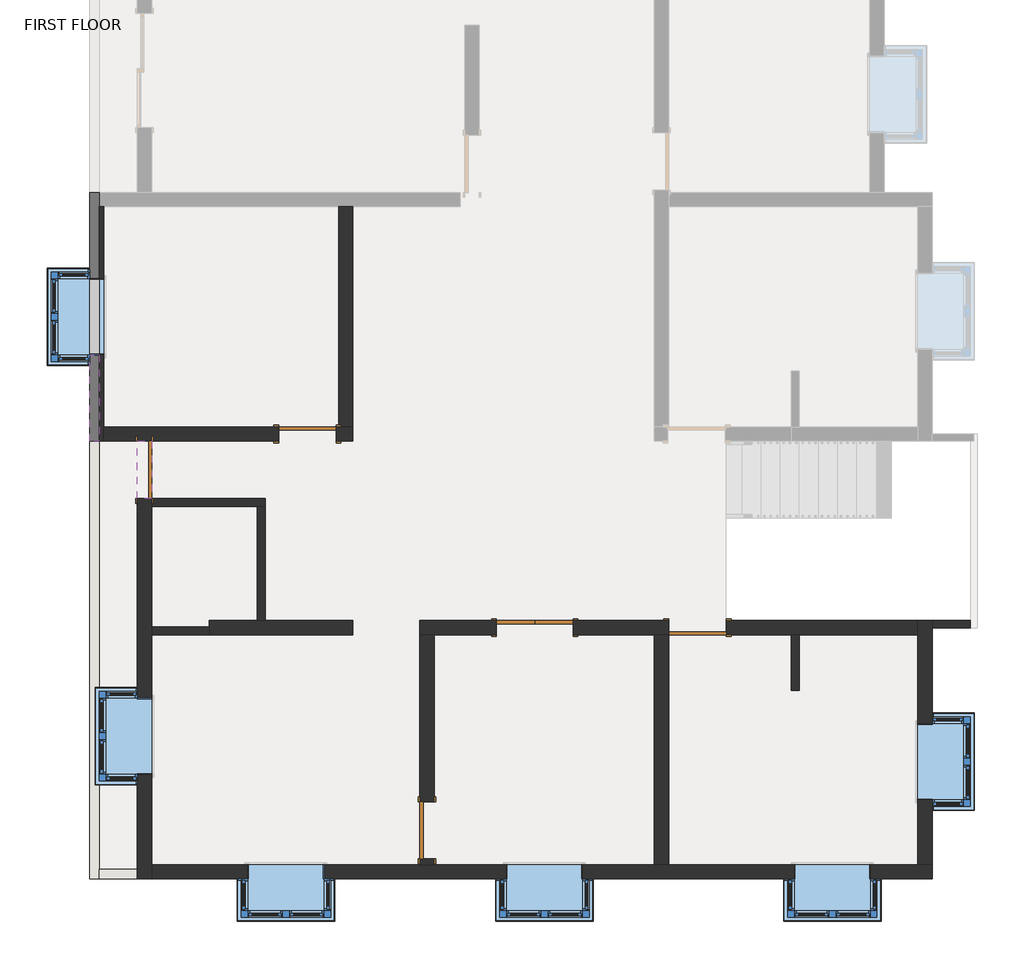
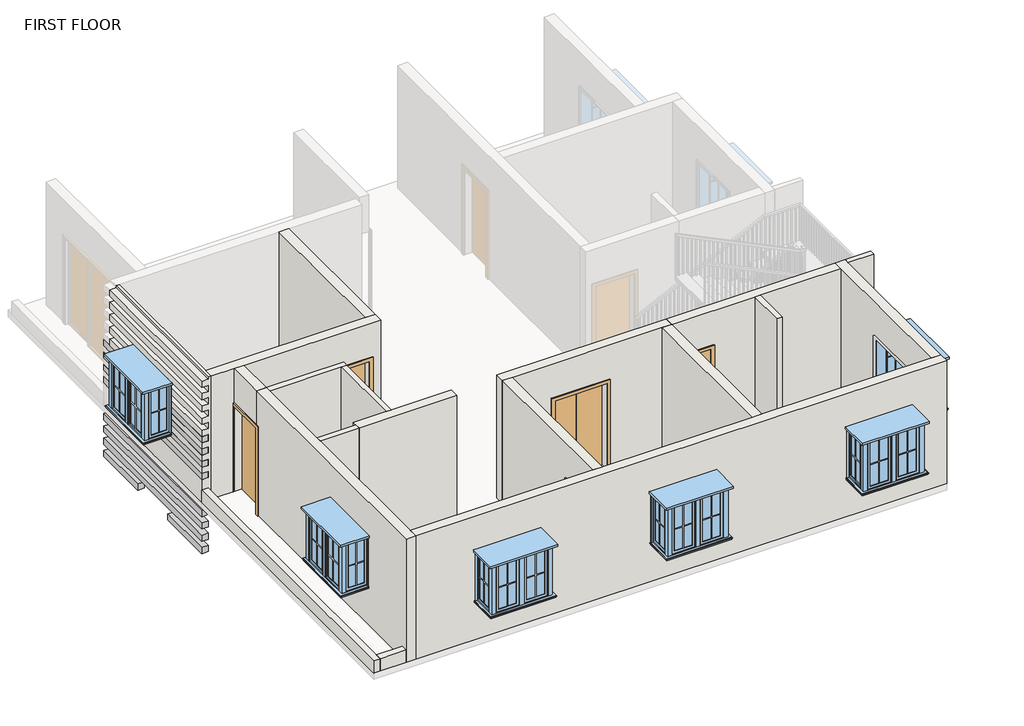
# One storey, part 1 of 6: 19 walls, 8 proxies, 6 windows, 5 doors.
"""IFC4 building model written with IfcOpenShell, lengths in millimetres."""

from ifc_helpers import new_model, si_unit, frame, origin, place, context, project, spatial, polyline, outline, extrude, faceted_brep, transform, mapped, element, save
from components import door_double_flush_panel_4_x7_7c704b5a, door_a90ba1ad, door_0ca8825f, window_bay_casement_box_90_degree_angle_4_x4_x2_07b705a1

model = new_model("IFC4")

# Units and contexts
model_context = context("Model", 3, world=origin())
ifc_project = project(units=[si_unit("LENGTHUNIT", "METRE", prefix="MILLI")], contexts=[model_context])

# Site, building, storey
site = spatial("IfcSite", under=ifc_project)
building = spatial("IfcBuilding", under=site)
storey = spatial("IfcBuildingStorey", under=building, Name="FIRST FLOOR", Elevation=3200.4)

# Proxies
placement = place(None, origin())
element("IfcBuildingElementProxy", 1, Name="Reveal", ObjectType="Reveal", at=placement, inside=storey, context=model_context, shape_type="SweptSolid", body=[
    extrude(outline(polyline([(-7008.3415084, 1592.333346), (-6855.9415084, 1592.333346), (-6855.9415084, 220.733346), (-7008.3415084, 220.733346), (-7008.3415084, 1592.333346)])), frame((0.0, 0.0, 1930.4), z_axis=(0.0, 0.0, 1.0), x_axis=(1.0, 0.0, 0.0)), (0.0, 0.0, 1.0), 152.4),
    extrude(outline(polyline([(-7008.3415084, 4183.133346), (-6855.9415084, 4183.133346), (-6855.9415084, 2811.533346), (-7008.3415084, 2811.533346), (-7008.3415084, 4183.133346)])), frame((0.0, 0.0, 1930.4), z_axis=(0.0, 0.0, 1.0), x_axis=(1.0, 0.0, 0.0)), (0.0, 0.0, 1.0), 152.4),
])
element("IfcBuildingElementProxy", 2, Name="Reveal", ObjectType="Reveal", at=placement, inside=storey, context=model_context, shape_type="SweptSolid", body=[
    extrude(outline(polyline([(-7008.3415084, 4183.133346), (-6855.9415084, 4183.133346), (-6855.9415084, 220.733346), (-7008.3415084, 220.733346), (-7008.3415084, 4183.133346)])), frame((0.0, 0.0, 2235.2), z_axis=(0.0, 0.0, 1.0), x_axis=(1.0, 0.0, 0.0)), (0.0, 0.0, 1.0), 152.4),
])
element("IfcBuildingElementProxy", 3, Name="Reveal", ObjectType="Reveal", at=placement, inside=storey, context=model_context, shape_type="SweptSolid", body=[
    extrude(outline(polyline([(-7008.3415084, 4183.133346), (-6855.9415084, 4183.133346), (-6855.9415084, 220.733346), (-7008.3415084, 220.733346), (-7008.3415084, 4183.133346)])), frame((0.0, 0.0, 2540.0), z_axis=(0.0, 0.0, 1.0), x_axis=(1.0, 0.0, 0.0)), (0.0, 0.0, 1.0), 152.4),
])
element("IfcBuildingElementProxy", 4, Name="Reveal", ObjectType="Reveal", at=placement, inside=storey, context=model_context, shape_type="SweptSolid", body=[
    extrude(outline(polyline([(-7008.3415084, 4183.133346), (-6855.9415084, 4183.133346), (-6855.9415084, 220.733346), (-7008.3415084, 220.733346), (-7008.3415084, 4183.133346)])), frame((0.0, 0.0, 2844.8), z_axis=(0.0, 0.0, 1.0), x_axis=(1.0, 0.0, 0.0)), (0.0, 0.0, 1.0), 152.4),
])
element("IfcBuildingElementProxy", 5, Name="Reveal", ObjectType="Reveal", at=placement, inside=storey, context=model_context, shape_type="SweptSolid", body=[
    extrude(outline(polyline([(-7008.3415084, 4183.133346), (-6855.9415084, 4183.133346), (-6855.9415084, 220.733346), (-7008.3415084, 220.733346), (-7008.3415084, 4183.133346)])), frame((0.0, 0.0, 3759.2), z_axis=(0.0, 0.0, 1.0), x_axis=(1.0, 0.0, 0.0)), (0.0, 0.0, 1.0), 152.4),
])
element("IfcBuildingElementProxy", 6, Name="Reveal", ObjectType="Reveal", at=placement, inside=storey, context=model_context, shape_type="SweptSolid", body=[
    extrude(outline(polyline([(-7008.3415084, 4183.133346), (-6855.9415084, 4183.133346), (-6855.9415084, 220.733346), (-7008.3415084, 220.733346), (-7008.3415084, 4183.133346)])), frame((0.0, 0.0, 4064.0), z_axis=(0.0, 0.0, 1.0), x_axis=(1.0, 0.0, 0.0)), (0.0, 0.0, 1.0), 152.4),
])
element("IfcBuildingElementProxy", 7, Name="Reveal", ObjectType="Reveal", at=placement, inside=storey, context=model_context, shape_type="SweptSolid", body=[
    extrude(outline(polyline([(-7008.3415084, 1592.333346), (-6855.9415084, 1592.333346), (-6855.9415084, 220.733346), (-7008.3415084, 220.733346), (-7008.3415084, 1592.333346)])), frame((0.0, 0.0, 4368.8), z_axis=(0.0, 0.0, 1.0), x_axis=(1.0, 0.0, 0.0)), (0.0, 0.0, 1.0), 152.4),
    extrude(outline(polyline([(-7008.3415084, 4183.133346), (-6855.9415084, 4183.133346), (-6855.9415084, 2811.533346), (-7008.3415084, 2811.533346), (-7008.3415084, 4183.133346)])), frame((0.0, 0.0, 4368.8), z_axis=(0.0, 0.0, 1.0), x_axis=(1.0, 0.0, 0.0)), (0.0, 0.0, 1.0), 152.4),
])
element("IfcBuildingElementProxy", 8, Name="Reveal", ObjectType="Reveal", at=placement, inside=storey, context=model_context, shape_type="SweptSolid", body=[
    extrude(outline(polyline([(-7008.3415084, 1592.333346), (-6855.9415084, 1592.333346), (-6855.9415084, 220.733346), (-7008.3415084, 220.733346), (-7008.3415084, 1592.333346)])), frame((0.0, 0.0, 4673.6), z_axis=(0.0, 0.0, 1.0), x_axis=(1.0, 0.0, 0.0)), (0.0, 0.0, 1.0), 152.4),
    extrude(outline(polyline([(-7008.3415084, 4183.133346), (-6855.9415084, 4183.133346), (-6855.9415084, 2811.533346), (-7008.3415084, 2811.533346), (-7008.3415084, 4183.133346)])), frame((0.0, 0.0, 4673.6), z_axis=(0.0, 0.0, 1.0), x_axis=(1.0, 0.0, 0.0)), (0.0, 0.0, 1.0), 152.4),
])

# Doors
door_double_flush_panel_4_x7_shape = door_double_flush_panel_4_x7_7c704b5a(model_context)
element("IfcDoor", 9, ObjectType="Door-Double-Flush_Panel : 4'x7'", at=placement, inside=storey, context=model_context, shape_type="MappedRepresentation", body=[
    mapped(door_double_flush_panel_4_x7_shape, transform((78.2584916, -2751.066654, 3200.4), x_axis=(1.0, 0.0, 0.0), y_axis=(0.0, 1.0, 0.0), z_axis=(0.0, 0.0, 1.0))),
])
door_shape = door_a90ba1ad(model_context)
element("IfcDoor", 10, ObjectType="Single-Flush : 36\" x 84\"", at=placement, inside=storey, context=model_context, shape_type="MappedRepresentation", body=[
    mapped(door_shape, transform((-1636.2415084, -5976.866654, 3200.4), x_axis=(0.0, -1.0, 0.0), y_axis=(1.0, 0.0, 0.0), z_axis=(0.0, 0.0, 1.0))),
])
door_2_shape = door_0ca8825f(model_context)
element("IfcDoor", 11, ObjectType="Single-Flush : 36\" x 84\"", at=placement, inside=storey, context=model_context, shape_type="MappedRepresentation", body=[
    mapped(door_2_shape, transform((-3541.2415084, 335.033346, 3200.4), x_axis=(1.0, 0.0, 0.0), y_axis=(0.0, 1.0, 0.0), z_axis=(0.0, 0.0, 1.0))),
])
element("IfcDoor", 12, ObjectType="Single-Flush : 36\" x 84\"", at=placement, inside=storey, context=model_context, shape_type="MappedRepresentation", body=[
    mapped(door_2_shape, transform((2669.0584916, -2751.066654, 3200.4), x_axis=(-1.0, 0.0, 0.0), y_axis=(0.0, -1.0, 0.0), z_axis=(0.0, 0.0, 1.0))),
])
element("IfcDoor", 13, ObjectType="Single-Flush : 36\" x 84\"", at=placement, inside=storey, context=model_context, shape_type="MappedRepresentation", body=[
    mapped(door_2_shape, transform((-6132.0415084, -236.466654, 3200.4), x_axis=(0.0, -1.0, 0.0), y_axis=(1.0, 0.0, 0.0), z_axis=(0.0, 0.0, 1.0))),
])

# Walls
element("IfcWall", 14, ObjectType="4.6\"", at=placement, inside=storey, context=model_context, shape_type="SweptSolid", body=[
    extrude(outline(polyline([(7009.1350459, -2753.606654), (6402.8584916, -2753.606654), (6402.8584916, -2636.766654), (7009.1350459, -2636.766654), (7009.1350459, -2753.606654)])), frame((0.0, 0.0, 3200.4), z_axis=(0.0, 0.0, 1.0), x_axis=(1.0, 0.0, 0.0)), (0.0, 0.0, 1.0), 3048.0),
])
element("IfcWall", 15, ObjectType="5\"", at=placement, inside=storey, context=model_context, shape_type="SweptSolid", body=[
    extrude(outline(polyline([(4159.1868368, -3751.826654), (4159.1868368, -2865.366654), (4286.1868368, -2865.366654), (4286.1868368, -3751.826654), (4159.1868368, -3751.826654)])), frame((0.0, 0.0, 3200.4), z_axis=(0.0, 0.0, 1.0), x_axis=(1.0, 0.0, 0.0)), (0.0, 0.0, 1.0), 3048.0),
])
element("IfcWall", 16, ObjectType="5\"", at=placement, inside=storey, context=model_context, shape_type="Brep", body=[
    faceted_brep([(-6017.7415084, -820.666654, 3200.4), (-4341.3415084, -820.666654, 3200.4), (-4214.3415084, -820.666654, 3200.4), (-4214.3415084, -820.666654, 6248.4), (-4341.3415084, -820.666654, 6248.4), (-6017.7415084, -820.666654, 6248.4), (-6017.7415084, -693.666654, 3200.4), (-6017.7415084, -693.666654, 6248.4), (-4214.3415084, -693.666654, 6248.4), (-4214.3415084, -693.666654, 3200.4)], [[[0, 1, 2, 3, 4, 5]], [[6, 7, 8, 9]], [[2, 1, 0, 6, 9]], [[5, 4, 3, 8, 7]], [[0, 5, 7, 6]], [[3, 2, 9, 8]]]),
])
element("IfcWall", 17, ObjectType="5\"", at=placement, inside=storey, context=model_context, shape_type="SweptSolid", body=[
    extrude(outline(polyline([(-4341.3415084, -2636.766654), (-4341.3415084, -820.666654), (-4214.3415084, -820.666654), (-4214.3415084, -2636.766654), (-4341.3415084, -2636.766654)])), frame((0.0, 0.0, 3200.4), z_axis=(0.0, 0.0, 1.0), x_axis=(1.0, 0.0, 0.0)), (0.0, 0.0, 1.0), 3048.0),
])
element("IfcWall", 18, ObjectType="5\"", at=placement, inside=storey, context=model_context, shape_type="SweptSolid", body=[
    extrude(outline(polyline([(-6017.7415084, -2738.366654), (-5103.3415084, -2738.366654), (-5103.3415084, -2865.366654), (-6017.7415084, -2865.366654), (-6017.7415084, -2738.366654)])), frame((0.0, 0.0, 3200.4), z_axis=(0.0, 0.0, 1.0), x_axis=(1.0, 0.0, 0.0)), (0.0, 0.0, 1.0), 3048.0),
])
element("IfcWall", 19, ObjectType="6\"", at=placement, inside=storey, context=model_context, shape_type="Brep", body=[
    faceted_brep([(-7008.3415084, 220.733346, 3200.4), (-7008.3415084, -6751.566654, 3200.4), (-7008.3415084, -6751.566654, 3505.2), (-7008.3415084, 220.733346, 3505.2), (-6855.9415084, 220.733346, 3200.4), (-6855.9415084, 220.733346, 3505.2), (-6855.9415084, -6599.166654, 3505.2), (-6855.9415084, -6751.566654, 3505.2), (-6855.9415084, -6751.566654, 3200.4), (-6855.9415084, -6599.166654, 3200.4)], [[[0, 1, 2, 3]], [[4, 5, 6, 7, 8, 9]], [[1, 0, 4, 9, 8]], [[3, 2, 7, 6, 5]], [[0, 3, 5, 4]], [[2, 1, 8, 7]]]),
])
element("IfcWall", 20, ObjectType="6\"", at=placement, inside=storey, context=model_context, shape_type="SweptSolid", body=[
    extrude(outline(polyline([(-6246.3415084, -6751.566654), (-6855.9415084, -6751.566654), (-6855.9415084, -6599.166654), (-6246.3415084, -6599.166654), (-6246.3415084, -6751.566654)])), frame((0.0, 0.0, 3200.4), z_axis=(0.0, 0.0, 1.0), x_axis=(1.0, 0.0, 0.0)), (0.0, 0.0, 1.0), 304.8),
])
element("IfcWall", 21, ObjectType="9\"", at=placement, inside=storey, context=model_context, shape_type="Brep", body=[
    faceted_brep([(-7008.3415084, 3954.533346, 3200.4), (-7008.3415084, 220.733346, 3200.4), (-7008.3415084, 220.733346, 3505.2), (-7008.3415084, 220.733346, 3759.2), (-7008.3415084, 3954.533346, 3759.2), (-7008.3415084, 2811.533346, 5384.8), (-7008.3415084, 1592.333346, 5384.8), (-7008.3415084, 1592.333346, 5435.6), (-7008.3415084, 220.733346, 5435.6), (-7008.3415084, 220.733346, 5588.0), (-7008.3415084, 3954.533346, 5588.0), (-7008.3415084, 3954.533346, 5435.6), (-7008.3415084, 2811.533346, 5435.6), (-7008.3415084, 220.733346, 6197.6), (-7008.3415084, 3954.533346, 6197.6), (-7008.3415084, 3954.533346, 6045.2), (-7008.3415084, 220.733346, 6045.2), (-7008.3415084, 220.733346, 5892.8), (-7008.3415084, 3954.533346, 5892.8), (-7008.3415084, 3954.533346, 5740.4), (-7008.3415084, 220.733346, 5740.4), (-7008.3415084, 220.733346, 5283.2), (-7008.3415084, 1592.333346, 5283.2), (-7008.3415084, 1592.333346, 5130.8), (-7008.3415084, 220.733346, 5130.8), (-7008.3415084, 2811.533346, 5283.2), (-7008.3415084, 3954.533346, 5283.2), (-7008.3415084, 3954.533346, 5130.8), (-7008.3415084, 2811.533346, 5130.8), (-7008.3415084, 220.733346, 4978.4), (-7008.3415084, 1592.333346, 4978.4), (-7008.3415084, 1592.333346, 4826.0), (-7008.3415084, 220.733346, 4826.0), (-7008.3415084, 2811.533346, 4978.4), (-7008.3415084, 3954.533346, 4978.4), (-7008.3415084, 3954.533346, 4826.0), (-7008.3415084, 2811.533346, 4826.0), (-7008.3415084, 220.733346, 4673.6), (-7008.3415084, 1592.333346, 4673.6), (-7008.3415084, 1592.333346, 4521.2), (-7008.3415084, 220.733346, 4521.2), (-7008.3415084, 2811.533346, 4673.6), (-7008.3415084, 3954.533346, 4673.6), (-7008.3415084, 3954.533346, 4521.2), (-7008.3415084, 2811.533346, 4521.2), (-7008.3415084, 220.733346, 4368.8), (-7008.3415084, 1592.333346, 4368.8), (-7008.3415084, 1592.333346, 4216.4), (-7008.3415084, 220.733346, 4216.4), (-7008.3415084, 2811.533346, 4368.8), (-7008.3415084, 3954.533346, 4368.8), (-7008.3415084, 3954.533346, 4216.4), (-7008.3415084, 2811.533346, 4216.4), (-7008.3415084, 220.733346, 4064.0), (-7008.3415084, 3954.533346, 4064.0), (-7008.3415084, 3954.533346, 3911.6), (-7008.3415084, 220.733346, 3911.6), (-6779.7415084, 220.733346, 3200.4), (-6779.7415084, 449.333346, 3200.4), (-6779.7415084, 3954.533346, 3200.4), (-6779.7415084, 3954.533346, 6248.4), (-6779.7415084, 449.333346, 6248.4), (-6779.7415084, 220.733346, 6248.4), (-6779.7415084, 2811.533346, 5384.8), (-6779.7415084, 2811.533346, 4114.8), (-6779.7415084, 1592.333346, 4114.8), (-6779.7415084, 1592.333346, 5384.8), (-6855.9415084, 220.733346, 3200.4), (-6855.9415084, 3954.533346, 6248.4), (-6855.9415084, 220.733346, 6248.4), (-6855.9415084, 2811.533346, 5384.8), (-6855.9415084, 2811.533346, 5283.2), (-6855.9415084, 2811.533346, 5130.8), (-6855.9415084, 2811.533346, 4978.4), (-6855.9415084, 2811.533346, 4826.0), (-6855.9415084, 2811.533346, 4673.6), (-6855.9415084, 2811.533346, 4521.2), (-6855.9415084, 2811.533346, 4368.8), (-6855.9415084, 2811.533346, 4216.4), (-6855.9415084, 2811.533346, 4114.8), (-6855.9415084, 1592.333346, 4114.8), (-6855.9415084, 1592.333346, 4216.4), (-6855.9415084, 1592.333346, 4368.8), (-6855.9415084, 1592.333346, 4521.2), (-6855.9415084, 1592.333346, 4673.6), (-6855.9415084, 1592.333346, 4826.0), (-6855.9415084, 1592.333346, 4978.4), (-6855.9415084, 1592.333346, 5130.8), (-6855.9415084, 1592.333346, 5283.2), (-6855.9415084, 1592.333346, 5384.8), (-6855.9415084, 3954.533346, 3759.2), (-6855.9415084, 3954.533346, 3911.6), (-6855.9415084, 3954.533346, 4064.0), (-6855.9415084, 3954.533346, 4216.4), (-6855.9415084, 3954.533346, 4368.8), (-6855.9415084, 3954.533346, 4521.2), (-6855.9415084, 3954.533346, 4673.6), (-6855.9415084, 3954.533346, 4826.0), (-6855.9415084, 3954.533346, 4978.4), (-6855.9415084, 3954.533346, 5130.8), (-6855.9415084, 3954.533346, 5283.2), (-6855.9415084, 3954.533346, 5435.6), (-6855.9415084, 3954.533346, 5588.0), (-6855.9415084, 3954.533346, 5740.4), (-6855.9415084, 3954.533346, 5892.8), (-6855.9415084, 3954.533346, 6045.2), (-6855.9415084, 3954.533346, 6197.6), (-6855.9415084, 220.733346, 6197.6), (-6855.9415084, 220.733346, 6045.2), (-6855.9415084, 220.733346, 5892.8), (-6855.9415084, 220.733346, 5740.4), (-6855.9415084, 220.733346, 5588.0), (-6855.9415084, 220.733346, 5435.6), (-6855.9415084, 220.733346, 5283.2), (-6855.9415084, 220.733346, 5130.8), (-6855.9415084, 220.733346, 4978.4), (-6855.9415084, 220.733346, 4826.0), (-6855.9415084, 220.733346, 4673.6), (-6855.9415084, 220.733346, 4521.2), (-6855.9415084, 220.733346, 4368.8), (-6855.9415084, 220.733346, 4216.4), (-6855.9415084, 220.733346, 4064.0), (-6855.9415084, 220.733346, 3911.6), (-6855.9415084, 220.733346, 3759.2), (-6855.9415084, 1592.333346, 5435.6), (-6855.9415084, 2811.533346, 5435.6)], [[[0, 1, 2, 3, 4]], [[5, 6, 7, 8, 9, 10, 11, 12]], [[13, 14, 15, 16]], [[17, 18, 19, 20]], [[21, 22, 23, 24]], [[25, 26, 27, 28]], [[29, 30, 31, 32]], [[33, 34, 35, 36]], [[37, 38, 39, 40]], [[41, 42, 43, 44]], [[45, 46, 47, 48]], [[49, 50, 51, 52]], [[53, 54, 55, 56]], [[57, 58, 59, 60, 61, 62], [63, 64, 65, 66]], [[1, 0, 59, 58, 57, 67]], [[62, 61, 60, 68, 69]], [[64, 63, 70, 71, 25, 28, 72, 73, 33, 36, 74, 75, 41, 44, 76, 77, 49, 52, 78, 79]], [[65, 64, 79, 80]], [[66, 65, 80, 81, 47, 46, 82, 83, 39, 38, 84, 85, 31, 30, 86, 87, 23, 22, 88, 89]], [[63, 66, 89, 6, 5, 70]], [[59, 0, 4, 90, 91, 55, 54, 92, 93, 51, 50, 94, 95, 43, 42, 96, 97, 35, 34, 98, 99, 27, 26, 100, 101, 11, 10, 102, 103, 19, 18, 104, 105, 15, 14, 106, 68, 60]], [[1, 67, 57, 62, 69, 107, 13, 16, 108, 109, 17, 20, 110, 111, 9, 8, 112, 113, 21, 24, 114, 115, 29, 32, 116, 117, 37, 40, 118, 119, 45, 48, 120, 121, 53, 56, 122, 123, 3, 2]], [[106, 107, 69, 68]], [[107, 106, 14, 13]], [[105, 108, 16, 15]], [[108, 105, 104, 109]], [[109, 104, 18, 17]], [[103, 110, 20, 19]], [[110, 103, 102, 111]], [[111, 102, 10, 9]], [[124, 7, 6, 89]], [[7, 124, 112, 8]], [[112, 124, 89, 88, 113]], [[113, 88, 22, 21]], [[12, 125, 70, 5]], [[125, 12, 11, 101]], [[70, 125, 101, 100, 71]], [[71, 100, 26, 25]], [[87, 114, 24, 23]], [[114, 87, 86, 115]], [[115, 86, 30, 29]], [[99, 72, 28, 27]], [[72, 99, 98, 73]], [[73, 98, 34, 33]], [[85, 116, 32, 31]], [[116, 85, 84, 117]], [[117, 84, 38, 37]], [[97, 74, 36, 35]], [[74, 97, 96, 75]], [[75, 96, 42, 41]], [[83, 118, 40, 39]], [[118, 83, 82, 119]], [[119, 82, 46, 45]], [[95, 76, 44, 43]], [[76, 95, 94, 77]], [[77, 94, 50, 49]], [[81, 120, 48, 47]], [[93, 78, 52, 51]], [[120, 81, 80, 79, 78, 93, 92, 121]], [[121, 92, 54, 53]], [[91, 122, 56, 55]], [[122, 91, 90, 123]], [[123, 90, 4, 3]]]),
])
element("IfcWall", 22, ObjectType="9\"", at=placement, inside=storey, context=model_context, shape_type="Brep", body=[
    faceted_brep([(-3084.0415084, 220.733346, 5334.0), (-3084.0415084, 220.733346, 3200.4), (-2817.3415084, 220.733346, 3200.4), (-2817.3415084, 220.733346, 6248.4), (-6017.7415084, 220.733346, 6248.4), (-6246.3415084, 220.733346, 6248.4), (-6779.7415084, 220.733346, 6248.4), (-6779.7415084, 220.733346, 3200.4), (-3998.4415084, 220.733346, 3200.4), (-3998.4415084, 220.733346, 5334.0), (-2817.3415084, 449.333346, 3200.4), (-3045.9415084, 449.333346, 3200.4), (-3084.0415084, 449.333346, 3200.4), (-3084.0415084, 449.333346, 5334.0), (-3998.4415084, 449.333346, 5334.0), (-3998.4415084, 449.333346, 3200.4), (-6779.7415084, 449.333346, 3200.4), (-6779.7415084, 449.333346, 6248.4), (-3045.9415084, 449.333346, 6248.4), (-2817.3415084, 449.333346, 6248.4)], [[[0, 1, 2, 3, 4, 5, 6, 7, 8, 9]], [[10, 11, 12, 13, 14, 15, 16, 17, 18, 19]], [[8, 7, 16, 15]], [[2, 1, 12, 11, 10]], [[6, 5, 4, 3, 19, 18, 17]], [[3, 2, 10, 19]], [[13, 12, 1, 0]], [[14, 13, 0, 9]], [[15, 14, 9, 8]], [[6, 17, 16, 7]]]),
])
element("IfcWall", 23, ObjectType="9\"", at=placement, inside=storey, context=model_context, shape_type="SweptSolid", body=[
    extrude(outline(polyline([(-2817.3415084, 3954.533346), (-2817.3415084, 449.333346), (-3045.9415084, 449.333346), (-3045.9415084, 3954.533346), (-2817.3415084, 3954.533346)])), frame((0.0, 0.0, 3200.4), z_axis=(0.0, 0.0, 1.0), x_axis=(1.0, 0.0, 0.0)), (0.0, 0.0, 1.0), 3048.0),
])
element("IfcWall", 24, ObjectType="9\"", at=placement, inside=storey, context=model_context, shape_type="Brep", body=[
    faceted_brep([(-6246.3415084, -693.666654, 3200.4), (-6246.3415084, -6599.166654, 3200.4), (-6246.3415084, -6751.566654, 3200.4), (-6246.3415084, -6751.566654, 3505.2), (-6246.3415084, -6751.566654, 6248.4), (-6246.3415084, -693.666654, 6248.4), (-6246.3415084, -693.666654, 5334.0), (-6246.3415084, -3868.666654, 5384.8), (-6246.3415084, -5087.866654, 5384.8), (-6246.3415084, -5087.866654, 4114.8), (-6246.3415084, -3868.666654, 4114.8), (-6017.7415084, -693.666654, 3200.4), (-6017.7415084, -693.666654, 5334.0), (-6017.7415084, -693.666654, 6248.4), (-6017.7415084, -820.666654, 6248.4), (-6017.7415084, -2738.366654, 6248.4), (-6017.7415084, -2865.366654, 6248.4), (-6017.7415084, -6522.966654, 6248.4), (-6017.7415084, -6751.566654, 6248.4), (-6017.7415084, -6751.566654, 3200.4), (-6017.7415084, -6522.966654, 3200.4), (-6017.7415084, -2865.366654, 3200.4), (-6017.7415084, -2738.366654, 3200.4), (-6017.7415084, -820.666654, 3200.4), (-6017.7415084, -3868.666654, 5384.8), (-6017.7415084, -3868.666654, 4114.8), (-6017.7415084, -5087.866654, 4114.8), (-6017.7415084, -5087.866654, 5384.8)], [[[0, 1, 2, 3, 4, 5, 6], [7, 8, 9, 10]], [[11, 12, 13, 14, 15, 16, 17, 18, 19, 20, 21, 22, 23], [24, 25, 26, 27]], [[2, 1, 0, 11, 23, 22, 21, 20, 19]], [[5, 4, 18, 17, 16, 15, 14, 13]], [[0, 6, 5, 13, 12, 11]], [[25, 24, 7, 10]], [[26, 25, 10, 9]], [[27, 26, 9, 8]], [[24, 27, 8, 7]], [[2, 19, 18, 4, 3]]]),
])
element("IfcWall", 25, ObjectType="9\"", at=placement, inside=storey, context=model_context, shape_type="Brep", body=[
    faceted_brep([(-2817.3415084, -2636.766654, 3200.4), (-4214.3415084, -2636.766654, 3200.4), (-4341.3415084, -2636.766654, 3200.4), (-5103.3415084, -2636.766654, 3200.4), (-5103.3415084, -2636.766654, 6248.4), (-4341.3415084, -2636.766654, 6248.4), (-4214.3415084, -2636.766654, 6248.4), (-2817.3415084, -2636.766654, 6248.4), (-2817.3415084, -2865.366654, 3200.4), (-2817.3415084, -2865.366654, 6248.4), (-5103.3415084, -2865.366654, 6248.4), (-5103.3415084, -2865.366654, 3200.4), (-5103.3415084, -2738.366654, 3200.4), (-5103.3415084, -2738.366654, 6248.4)], [[[0, 1, 2, 3, 4, 5, 6, 7]], [[8, 9, 10, 11]], [[3, 2, 1, 0, 8, 11, 12]], [[4, 3, 12, 11, 10, 13]], [[7, 6, 5, 4, 13, 10, 9]], [[0, 7, 9, 8]]]),
])
element("IfcWall", 26, ObjectType="9\"", at=placement, inside=storey, context=model_context, shape_type="Brep", body=[
    faceted_brep([(2211.8584916, -2865.366654, 6248.4), (1983.2584916, -2865.366654, 6248.4), (-1521.9415084, -2865.366654, 6248.4), (-1750.5415084, -2865.366654, 6248.4), (-1750.5415084, -2865.366654, 3200.4), (-1521.9415084, -2865.366654, 3200.4), (-531.3415084, -2865.366654, 3200.4), (-531.3415084, -2865.366654, 5334.0), (687.8584916, -2865.366654, 5334.0), (687.8584916, -2865.366654, 3200.4), (1983.2584916, -2865.366654, 3200.4), (2211.8584916, -2865.366654, 3200.4), (2211.8584916, -2865.366654, 5334.0), (-1750.5415084, -2636.766654, 6248.4), (2211.8584916, -2636.766654, 6248.4), (2211.8584916, -2636.766654, 5334.0), (2211.8584916, -2636.766654, 3200.4), (687.8584916, -2636.766654, 3200.4), (687.8584916, -2636.766654, 5334.0), (-531.3415084, -2636.766654, 5334.0), (-531.3415084, -2636.766654, 3200.4), (-1750.5415084, -2636.766654, 3200.4)], [[[0, 1, 2, 3, 4, 5, 6, 7, 8, 9, 10, 11, 12]], [[13, 14, 15, 16, 17, 18, 19, 20, 21]], [[16, 11, 10, 9, 17]], [[4, 21, 20, 6, 5]], [[3, 2, 1, 0, 14, 13]], [[0, 12, 11, 16, 15, 14]], [[4, 3, 13, 21]], [[8, 18, 17, 9]], [[18, 8, 7, 19]], [[19, 7, 6, 20]]]),
])
element("IfcWall", 27, ObjectType="9\"", at=placement, inside=storey, context=model_context, shape_type="SweptSolid", body=[
    extrude(outline(polyline([(1983.2584916, -6522.966654), (1983.2584916, -2865.366654), (2211.8584916, -2865.366654), (2211.8584916, -6522.966654), (1983.2584916, -6522.966654)])), frame((0.0, 0.0, 3200.4), z_axis=(0.0, 0.0, 1.0), x_axis=(1.0, 0.0, 0.0)), (0.0, 0.0, 1.0), 3048.0),
])
element("IfcWall", 28, ObjectType="9\"", at=placement, inside=storey, context=model_context, shape_type="Brep", body=[
    faceted_brep([(-6017.7415084, -6751.566654, 6248.4), (-6017.7415084, -6751.566654, 3200.4), (6402.8584916, -6751.566654, 3200.4), (6402.8584916, -6751.566654, 6248.4), (-378.9415084, -6751.566654, 5384.8), (840.2584916, -6751.566654, 5384.8), (840.2584916, -6751.566654, 4114.8), (-378.9415084, -6751.566654, 4114.8), (4205.7584916, -6751.566654, 5384.8), (5424.9584916, -6751.566654, 5384.8), (5424.9584916, -6751.566654, 4114.8), (4205.7584916, -6751.566654, 4114.8), (-4493.7415084, -6751.566654, 5384.8), (-3274.5415084, -6751.566654, 5384.8), (-3274.5415084, -6751.566654, 4114.8), (-4493.7415084, -6751.566654, 4114.8), (-6017.7415084, -6522.966654, 3200.4), (-6017.7415084, -6522.966654, 6248.4), (-1750.5415084, -6522.966654, 6248.4), (-1521.9415084, -6522.966654, 6248.4), (1983.2584916, -6522.966654, 6248.4), (2211.8584916, -6522.966654, 6248.4), (6174.2584916, -6522.966654, 6248.4), (6402.8584916, -6522.966654, 6248.4), (6402.8584916, -6522.966654, 3200.4), (6174.2584916, -6522.966654, 3200.4), (2211.8584916, -6522.966654, 3200.4), (1983.2584916, -6522.966654, 3200.4), (-1521.9415084, -6522.966654, 3200.4), (-1750.5415084, -6522.966654, 3200.4), (-378.9415084, -6522.966654, 5384.8), (-378.9415084, -6522.966654, 4114.8), (840.2584916, -6522.966654, 4114.8), (840.2584916, -6522.966654, 5384.8), (4205.7584916, -6522.966654, 5384.8), (4205.7584916, -6522.966654, 4114.8), (5424.9584916, -6522.966654, 4114.8), (5424.9584916, -6522.966654, 5384.8), (-4493.7415084, -6522.966654, 5384.8), (-4493.7415084, -6522.966654, 4114.8), (-3274.5415084, -6522.966654, 4114.8), (-3274.5415084, -6522.966654, 5384.8)], [[[0, 1, 2, 3], [4, 5, 6, 7], [8, 9, 10, 11], [12, 13, 14, 15]], [[16, 17, 18, 19, 20, 21, 22, 23, 24, 25, 26, 27, 28, 29], [30, 31, 32, 33], [34, 35, 36, 37], [38, 39, 40, 41]], [[2, 1, 16, 29, 28, 27, 26, 25, 24]], [[0, 3, 23, 22, 21, 20, 19, 18, 17]], [[3, 2, 24, 23]], [[31, 30, 4, 7]], [[32, 31, 7, 6]], [[33, 32, 6, 5]], [[30, 33, 5, 4]], [[35, 34, 8, 11]], [[36, 35, 11, 10]], [[37, 36, 10, 9]], [[34, 37, 9, 8]], [[39, 38, 12, 15]], [[40, 39, 15, 14]], [[41, 40, 14, 13]], [[38, 41, 13, 12]], [[0, 17, 16, 1]]]),
])
element("IfcWall", 29, ObjectType="9\"", at=placement, inside=storey, context=model_context, shape_type="Brep", body=[
    faceted_brep([(6402.8584916, -6522.966654, 3200.4), (6402.8584916, -2753.606654, 3200.4), (6402.8584916, -2636.766654, 3200.4), (6402.8584916, -2636.766654, 6248.4), (6402.8584916, -2753.606654, 6248.4), (6402.8584916, -6522.966654, 6248.4), (6402.8584916, -5494.266654, 5384.8), (6402.8584916, -4275.066654, 5384.8), (6402.8584916, -4275.066654, 4114.8), (6402.8584916, -5494.266654, 4114.8), (6174.2584916, -6522.966654, 3200.4), (6174.2584916, -6522.966654, 6248.4), (6174.2584916, -2865.366654, 6248.4), (6174.2584916, -2636.766654, 6248.4), (6174.2584916, -2636.766654, 3200.4), (6174.2584916, -2865.366654, 3200.4), (6174.2584916, -5494.266654, 5384.8), (6174.2584916, -5494.266654, 4114.8), (6174.2584916, -4275.066654, 4114.8), (6174.2584916, -4275.066654, 5384.8)], [[[0, 1, 2, 3, 4, 5], [6, 7, 8, 9]], [[10, 11, 12, 13, 14, 15], [16, 17, 18, 19]], [[2, 1, 0, 10, 15, 14]], [[5, 4, 3, 13, 12, 11]], [[0, 5, 11, 10]], [[3, 2, 14, 13]], [[17, 16, 6, 9]], [[18, 17, 9, 8]], [[19, 18, 8, 7]], [[16, 19, 7, 6]]]),
])
element("IfcWall", 30, ObjectType="9\"", at=placement, inside=storey, context=model_context, shape_type="Brep", body=[
    faceted_brep([(2211.8584916, -2636.766654, 6248.4), (6174.2584916, -2636.766654, 6248.4), (6174.2584916, -2636.766654, 3200.4), (3126.2584916, -2636.766654, 3200.4), (3126.2584916, -2636.766654, 5334.0), (2211.8584916, -2636.766654, 5334.0), (6174.2584916, -2865.366654, 6248.4), (4286.1868368, -2865.366654, 6248.4), (4159.1868368, -2865.366654, 6248.4), (2211.8584916, -2865.366654, 6248.4), (2211.8584916, -2865.366654, 5334.0), (3126.2584916, -2865.366654, 5334.0), (3126.2584916, -2865.366654, 3200.4), (4159.1868368, -2865.366654, 3200.4), (4286.1868368, -2865.366654, 3200.4), (6174.2584916, -2865.366654, 3200.4)], [[[0, 1, 2, 3, 4, 5]], [[6, 7, 8, 9, 10, 11, 12, 13, 14, 15]], [[2, 15, 14, 13, 12, 3]], [[1, 0, 9, 8, 7, 6]], [[2, 1, 6, 15]], [[9, 0, 5, 10]], [[4, 11, 10, 5]], [[11, 4, 3, 12]]]),
])
element("IfcWall", 31, ObjectType="9\"", at=placement, inside=storey, context=model_context, shape_type="SweptSolid", body=[
    extrude(outline(polyline([(-6434.066654, 5334.0), (-6434.066654, 3200.4), (-6522.966654, 3200.4), (-6522.966654, 6248.4), (-2865.366654, 6248.4), (-2865.366654, 3200.4), (-5519.666654, 3200.4), (-5519.666654, 5334.0), (-6434.066654, 5334.0)])), frame((-1750.5415084, 0.0, 0.0), z_axis=(1.0, 0.0, 0.0), x_axis=(0.0, 1.0, 0.0)), (0.0, 0.0, 1.0), 228.6),
])
element("IfcWall", 32, ObjectType="9\"", at=placement, inside=storey, context=model_context, shape_type="SweptSolid", body=[
    extrude(outline(polyline([(-6017.7415084, 220.733346), (-6017.7415084, -693.666654), (-6246.3415084, -693.666654), (-6246.3415084, 220.733346), (-6017.7415084, 220.733346)])), frame((0.0, 0.0, 5334.0), z_axis=(0.0, 0.0, 1.0), x_axis=(1.0, 0.0, 0.0)), (0.0, 0.0, 1.0), 914.4),
])

# Windows
window_bay_casement_box_90_degree_angle_4_x4_x2_shape = window_bay_casement_box_90_degree_angle_4_x4_x2_07b705a1(model_context)
element("IfcWindow", 33, ObjectType="Window-Bay-Casement-Box-90_Degree_Angle : 4'X4'X2'", at=placement, inside=storey, context=model_context, shape_type="MappedRepresentation", body=[
    mapped(window_bay_casement_box_90_degree_angle_4_x4_x2_shape, transform((-6894.0415084, 2201.933346, 3505.2), x_axis=(0.0, 1.0, 0.0), y_axis=(-1.0, 0.0, 0.0), z_axis=(0.0, 0.0, 1.0))),
])
element("IfcWindow", 34, ObjectType="Window-Bay-Casement-Box-90_Degree_Angle : 4'X4'X2'", at=placement, inside=storey, context=model_context, shape_type="MappedRepresentation", body=[
    mapped(window_bay_casement_box_90_degree_angle_4_x4_x2_shape, transform((-6132.0415084, -4478.266654, 3505.2), x_axis=(0.0, 1.0, 0.0), y_axis=(-1.0, 0.0, 0.0), z_axis=(0.0, 0.0, 1.0))),
])
element("IfcWindow", 35, ObjectType="Window-Bay-Casement-Box-90_Degree_Angle : 4'X4'X2'", at=placement, inside=storey, context=model_context, shape_type="MappedRepresentation", body=[
    mapped(window_bay_casement_box_90_degree_angle_4_x4_x2_shape, transform((6288.5584916, -4884.666654, 3505.2), x_axis=(0.0, -1.0, 0.0), y_axis=(1.0, 0.0, 0.0), z_axis=(0.0, 0.0, 1.0))),
])
element("IfcWindow", 36, ObjectType="Window-Bay-Casement-Box-90_Degree_Angle : 4'X4'X2'", at=placement, inside=storey, context=model_context, shape_type="MappedRepresentation", body=[
    mapped(window_bay_casement_box_90_degree_angle_4_x4_x2_shape, transform((230.6584916, -6637.266654, 3505.2), x_axis=(-1.0, 0.0, 0.0), y_axis=(0.0, -1.0, 0.0), z_axis=(0.0, 0.0, 1.0))),
])
element("IfcWindow", 37, ObjectType="Window-Bay-Casement-Box-90_Degree_Angle : 4'X4'X2'", at=placement, inside=storey, context=model_context, shape_type="MappedRepresentation", body=[
    mapped(window_bay_casement_box_90_degree_angle_4_x4_x2_shape, transform((4815.3584916, -6637.266654, 3505.2), x_axis=(-1.0, 0.0, 0.0), y_axis=(0.0, -1.0, 0.0), z_axis=(0.0, 0.0, 1.0))),
])
element("IfcWindow", 38, ObjectType="Window-Bay-Casement-Box-90_Degree_Angle : 4'X4'X2'", at=placement, inside=storey, context=model_context, shape_type="MappedRepresentation", body=[
    mapped(window_bay_casement_box_90_degree_angle_4_x4_x2_shape, transform((-3884.1415084, -6637.266654, 3505.2), x_axis=(-1.0, 0.0, 0.0), y_axis=(0.0, -1.0, 0.0), z_axis=(0.0, 0.0, 1.0))),
])

save(model, "model.ifc")

# Revit data of these elements
# Type "Door-Double-Flush_Panel : 4'x7'"
#   Type Mark = "9"
#   Construction Type Id = "DOOR"
#   Assembly Code = "C1020"
#   Analytic Construction = "Wooden"
#   Thickness = 0' - 2"
#   Thermal Resistance (R) = 2.5876 (h·ft²·°F)/BTU
#   Swing Angle [instance default] = 90.00°
#   Panel Width = 2' - 0"
#   Heat Transfer Coefficient (U) = 0.3865 BTU/(h·ft²·°F)
#   Height = 7' - 0"
#   Trim Projection Ext = 0' - 1"
#   Trim Projection Int = 0' - 1"
#   Trim Width = 0' - 3"
#   Width = 4' - 0"
#   Define Thermal Properties by = 1
#   Panel Material = Wood - Birch - Solid Stained Light Low Gloss
#   Trim Material = Paint - Sienna
#   Visual Light Transmittance = 0
#   Solar Heat Gain Coefficient = 0
#   Function = (empty or 0)
#   Wall Closure = (empty or 0)
# Type "Single-Flush : 36\" x 84\""
#   Type Mark = "1"
#   Construction Type Id = "MDOOR"
#   Assembly Code = "C1020"
#   Analytic Construction = "Metal"
#   Thickness = 0' - 2"
#   Heat Transfer Coefficient (U) = 0.651978 BTU/(h·ft²·°F)
#   Height = 7' - 0"
#   Trim Projection Ext = 0' - 1"
#   Trim Projection Int = 0' - 1"
#   Trim Width = 0' - 3"
#   Width = 3' - 0"
#   Define Thermal Properties by = 1
#   Define Thermal Properties by = 1
#   Door Material = Door - Panel
#   Frame Material = Door - Frame
#   Visual Light Transmittance = 0
#   Solar Heat Gain Coefficient = 0
#   Function = (empty or 0)
#   Wall Closure = (empty or 0)
# Type "4.6\""
#   Assembly Code = "B2010"
#   Layers, outside or top first: 0' - 4 77/128" no material (function 1)
# Type "5\""
#   Assembly Code = "B2010"
#   Layers, outside or top first: 0' - 5" no material (function 1)
# Type "6\""
#   Assembly Code = "B2010"
#   Layers, outside or top first: 0' - 6" no material (function 1)
# Type "9\""
#   Assembly Code = "B2010"
#   Layers, outside or top first: 0' - 9" "WALL 1" (function 1)
# Type "Window-Bay-Casement-Box-90_Degree_Angle : 4'X4'X2'"
#   Type Mark = "20"
#   Fire Rating = "0.5h"
#   Assembly Code = "B2020100"
#   Analytic Construction = "1/8 in Pilkington single glazing"
#   Width = 4' - 0"
#   Wall Thickness [instance default] = 0' - 6"
#   Visual Light Transmittance = 0.9
#   Trim Width = 4' - 8"
#   Trim Height = 4' - 0"
#   Thermal Resistance (R) = 1.5394 (h·ft²·°F)/BTU
#   Solar Heat Gain Coefficient = 0.86
#   Rough Width = 4' - 0 1/2"
#   Rough Height = 4' - 0 1/2"
#   Height 1 = 4' - 2"
#   Height = 4' - 0"
#   Heat Transfer Coefficient (U) = 0.6496 BTU/(h·ft²·°F)
#   Depth = 2' - 0"
#   Default Sill Height = 2' - 0"
#   Muntin Visibility = yes
#   Interior Trim Visibility [instance default] = yes
#   Exterior Trim Visibility [instance default] = yes
#   Muntin Pattern = Muntin Pattern_2x2 : Muntin Pattern_2x2
#   Interior Trim Material = Wood - Stained
#   Exterior Trim Material = Clad - White
#   Exterior Trim = element 423684
#   Interior Trim = Trim-Window-Interior-Flat : Picture Frame
#   Interior Frame Material = Wood - Stained
#   Glass Panel Material = Glass
#   Exterior Frame Material = Clad - White
#   Wall Closure = (empty or 0)
# Element 9 (IfcDoor, "Door-Double-Flush_Panel : 4'x7'")
#   Swing Angle = 90.00°
#   Phase Created = New Construction
#   Materials on its faces: "Paint - Sienna", "Wood - Birch - Solid Stained Light Low Gloss"
# Elements 10, 11, 12, 13 (IfcDoor, "Single-Flush : 36\" x 84\"")
#   Phase Created = New Construction
#   Materials on its faces: "Door - Frame", "Door - Panel"
# Element 14 (IfcWall, "4.6\"")
#   Top Offset = -0' - 6"
#   Base Offset = 0' - 0"
#   wall height = 10' - 0"
#   Phase Created = New Construction
#   Base Constraint = FIRST FLOOR
#   Top Constraint = SECOND FLOOR
#   Materials on its faces: "Default Wall", "WALL 1"
# Elements 15, 16, 17, 18 (IfcWall, "5\"")
#   Top Offset = -0' - 6"
#   Base Offset = 0' - 0"
#   wall height = 10' - 0"
#   Phase Created = New Construction
#   Base Constraint = FIRST FLOOR
#   Top Constraint = SECOND FLOOR
#   Materials on its faces: "Default Wall"
# Elements 19, 20 (IfcWall, "6\"")
#   Top Offset = -0' - 6"
#   Base Offset = 0' - 0"
#   Unconnected Height = 1' - 0"
#   wall height = 1' - 0"
#   Phase Created = New Construction
#   Base Constraint = FIRST FLOOR
#   Materials on its faces: "Default Wall", "WALL 4"
# Elements 21, 28 (IfcWall, "9\"")
#   Top Offset = -0' - 6"
#   Base Offset = 0' - 0"
#   wall height = 10' - 0"
#   Phase Created = New Construction
#   Base Constraint = FIRST FLOOR
#   Top Constraint = SECOND FLOOR
#   Materials on its faces: "WALL 1", "WALL 2"
# Elements 22, 23, 25, 26, 27, 29, 30, 31, 32 (IfcWall, "9\"")
#   Top Offset = -0' - 6"
#   Base Offset = 0' - 0"
#   wall height = 10' - 0"
#   Phase Created = New Construction
#   Base Constraint = FIRST FLOOR
#   Top Constraint = SECOND FLOOR
#   Materials on its faces: "WALL 1"
# Element 24 (IfcWall, "9\"")
#   Top Offset = -0' - 6"
#   Base Offset = 0' - 0"
#   wall height = 10' - 0"
#   Phase Created = New Construction
#   Base Constraint = FIRST FLOOR
#   Top Constraint = SECOND FLOOR
#   Materials on its faces: "WALL 1", "Default Wall", "WALL 2"
# Element 33 (IfcWindow, "Window-Bay-Casement-Box-90_Degree_Angle : 4'X4'X2'")
#   Mark = "17"
#   Phase Created = New Construction
#   Materials on its faces: "Clad - White", "Wood - Stained", "Glass"
# Element 34 (IfcWindow, "Window-Bay-Casement-Box-90_Degree_Angle : 4'X4'X2'")
#   Mark = "18"
#   Phase Created = New Construction
#   Materials on its faces: "Clad - White", "Wood - Stained", "Glass"
# Element 35 (IfcWindow, "Window-Bay-Casement-Box-90_Degree_Angle : 4'X4'X2'")
#   Mark = "19"
#   Phase Created = New Construction
#   Materials on its faces: "Clad - White", "Wood - Stained", "Glass"
# Element 36 (IfcWindow, "Window-Bay-Casement-Box-90_Degree_Angle : 4'X4'X2'")
#   Mark = "24"
#   Phase Created = New Construction
#   Materials on its faces: "Clad - White", "Wood - Stained", "Glass"
# Element 37 (IfcWindow, "Window-Bay-Casement-Box-90_Degree_Angle : 4'X4'X2'")
#   Mark = "25"
#   Phase Created = New Construction
#   Materials on its faces: "Clad - White", "Wood - Stained", "Glass"
# Element 38 (IfcWindow, "Window-Bay-Casement-Box-90_Degree_Angle : 4'X4'X2'")
#   Mark = "26"
#   Phase Created = New Construction
#   Materials on its faces: "Clad - White", "Wood - Stained", "Glass"
# Materials
#   "Wood - Birch - Solid Stained Light Low Gloss": class "Wood", colour RGB 210 159 95, transparency 0, Cost = 0
#   "Paint - Sienna": colour RGB 118 70 51, transparency 0, Cost = 0
#   "Door - Panel": class "Wood", colour RGB 210 159 95, transparency 0, Cost = 0
#   "Door - Frame": colour RGB 118 70 51, transparency 0, Cost = 0
#   "WALL 1": class "Generic", colour RGB 233 224 215, transparency 0, Cost = 0
#   "Wood - Stained": class "Wood", colour RGB 224 178 126, transparency 0, Cost = 0
#   "Clad - White": class "Wood", colour RGB 242 242 238, transparency 0, Cost = 0
#   "Glass": class "Glass", colour RGB 0 128 192, transparency 0.75, Description = "Soda Lime Glass", Cost = 0
#   "Default Wall": colour RGB 128 128 128, transparency 0, Cost = 0
#   "WALL 4": class "Generic", colour RGB 32 32 32, transparency 0, Cost = 0
#   "WALL 2": class "Generic", colour RGB 52 58 64, transparency 0, Cost = 0
